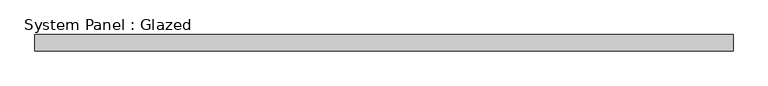
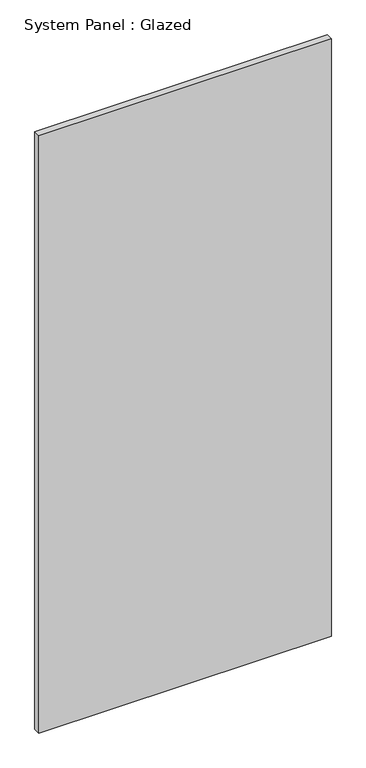
"""IFC4 building model written with IfcOpenShell, lengths in millimetres: plate geometry, System Panel : Glazed."""

from ifc_helpers import new_model, si_unit, origin, origin_with_axes, place, context, project, spatial, polyline, outline, extrude, source, transform, mapped, element, save


def system_panel_glazed_91cb7ab6(model_context):
    return source(origin(), model_context, "Body", "SweptSolid", [
        extrude(outline(polyline([(542.9250001, 19.05), (-542.9250001, 19.05), (-542.9250001, 44.45), (542.9250001, 44.45), (542.9250001, 19.05)])), origin_with_axes(), (0.0, 0.0, 1.0), 2343.15),
    ])


if __name__ == "__main__":
    model = new_model("IFC4")
    model_context = context("Model", 3, world=origin())
    ifc_project = project(units=[si_unit("LENGTHUNIT", "METRE", prefix="MILLI")], contexts=[model_context])
    site = spatial("IfcSite", under=ifc_project)
    building = spatial("IfcBuilding", under=site)
    placement = place(None, origin())
    system_panel_glazed_shape = system_panel_glazed_91cb7ab6(model_context)
    element("IfcPlate", 1, ObjectType="System Panel : Glazed", at=placement, inside=building, context=model_context, shape_type="MappedRepresentation", body=[
        mapped(system_panel_glazed_shape, transform((0.0, 0.0, 0.0), x_axis=(1.0, 0.0, 0.0), y_axis=(0.0, 1.0, 0.0), z_axis=(0.0, 0.0, 1.0))),
    ])
    save(model, "model.ifc")

# Revit data of these elements
# Type "System Panel : Glazed"
#   Construction Type Id = "GSP4R"
#   Analytic Construction = "1/8 in Pilkington single glazing"
#   Visual Light Transmittance = 0.9
#   Solar Heat Gain Coefficient = 0.86
#   Heat Transfer Coefficient (U) = 1.18115 BTU/(h·ft²·°F)
#   Define Thermal Properties by = 1
# Element 1 (IfcPlate, "System Panel : Glazed")
#   Materials on its faces: "Glass"
# Materials
#   "Glass": class "Glass", colour RGB 0 128 192, transparency 0.75, Description = "Soda Lime Glass", Cost = 0
